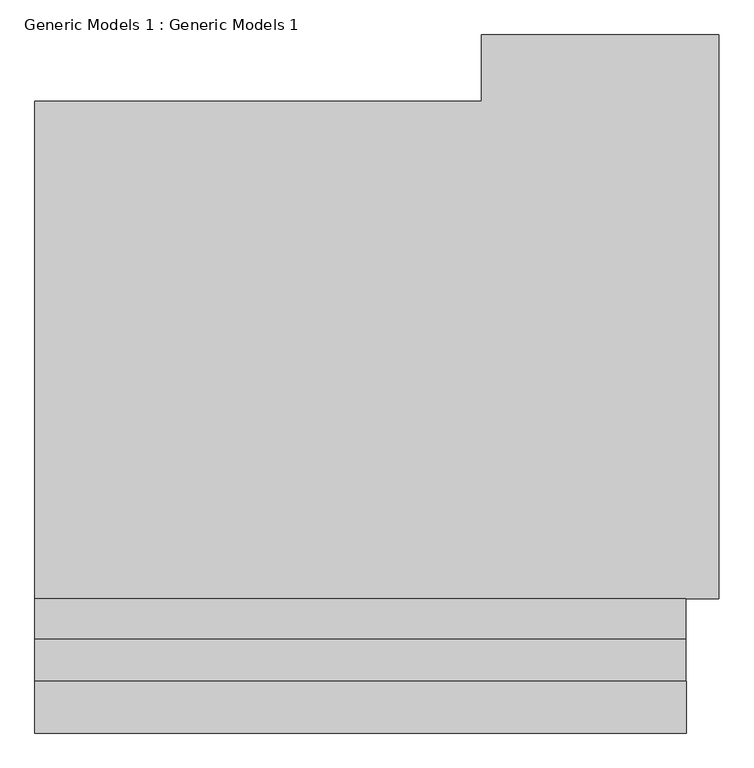
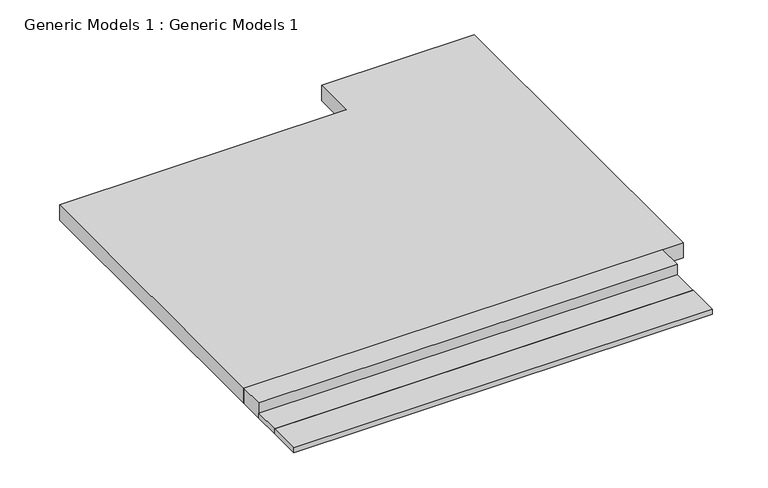
"""IFC4 building model written with IfcOpenShell, lengths in millimetres: proxy geometry, Generic Models 1 : Generic Models 1."""

from ifc_helpers import new_model, si_unit, origin, origin_with_axes, place, context, project, spatial, polyline, outline, extrude, faceted_brep, source, transform, mapped, element, save


def generic_models_1_generic_models_1_8617edb6(model_context):
    return source(origin(), model_context, "Body", "SolidModel", [
        extrude(outline(polyline([(-3404.2569605, -13729.0338546), (-11243.5120831, -13729.0338546), (-11243.5120831, -13107.5657682), (-3404.2569605, -13107.5657682), (-3404.2569605, -13729.0338546)])), origin_with_axes(), (0.0, 0.0, 1.0), 98.2270407),
        extrude(outline(polyline([(-3407.6218413, -13107.5657682), (-11243.5120831, -13107.5657682), (-11243.5120831, -12592.2491176), (-3407.6218413, -12592.2491176), (-3407.6218413, -13107.5657682)])), origin_with_axes(), (0.0, 0.0, 1.0), 98.2270407),
        extrude(outline(polyline([(-3406.8525483, -12592.2491176), (-11243.5120831, -12592.2491176), (-11243.5120831, -12113.2945627), (-3406.8525483, -12113.2945627), (-3406.8525483, -12592.2491176)])), origin_with_axes(), (0.0, 0.0, 1.0), 304.8),
        faceted_brep([(-11243.5120831, -12113.2945627, 0.0), (-3013.9120831, -12113.2945627, 0.0), (-3013.9120831, -12113.2945627, 304.7291805), (-11243.5120831, -12113.2945627, 304.7291805), (-11243.5120831, -6131.5945627, 0.0), (-11243.5120831, -6131.5945627, 304.7291805), (-5871.4120831, -6131.5945627, 304.7291805), (-5871.4120831, -6131.5945627, 0.0), (-5871.4120831, -5331.4945627, 0.0), (-3013.9120831, -5331.4945627, 0.0), (-3013.9120831, -5331.4945627, 304.8), (-5871.4120831, -5331.4945627, 304.7291805)], [[[0, 1, 2, 3]], [[4, 5, 6, 7]], [[1, 0, 4, 7, 8, 9]], [[2, 1, 9, 10]], [[3, 2, 10, 11, 6, 5]], [[0, 3, 5, 4]], [[11, 10, 9, 8]], [[6, 11, 8, 7]]]),
    ])


if __name__ == "__main__":
    model = new_model("IFC4")
    model_context = context("Model", 3, world=origin())
    ifc_project = project(units=[si_unit("LENGTHUNIT", "METRE", prefix="MILLI")], contexts=[model_context])
    site = spatial("IfcSite", under=ifc_project)
    building = spatial("IfcBuilding", under=site)
    placement = place(None, origin())
    generic_models_1_generic_models_1_shape = generic_models_1_generic_models_1_8617edb6(model_context)
    element("IfcBuildingElementProxy", 1, Name="Generic Models 1 : Generic Models 1", ObjectType="Generic Models 1 : Generic Models 1", at=placement, inside=building, context=model_context, shape_type="MappedRepresentation", body=[
        mapped(generic_models_1_generic_models_1_shape, transform((0.0, 0.0, 0.0), x_axis=(1.0, 0.0, 0.0), y_axis=(0.0, 1.0, 0.0), z_axis=(0.0, 0.0, 1.0))),
    ])
    save(model, "model.ifc")
